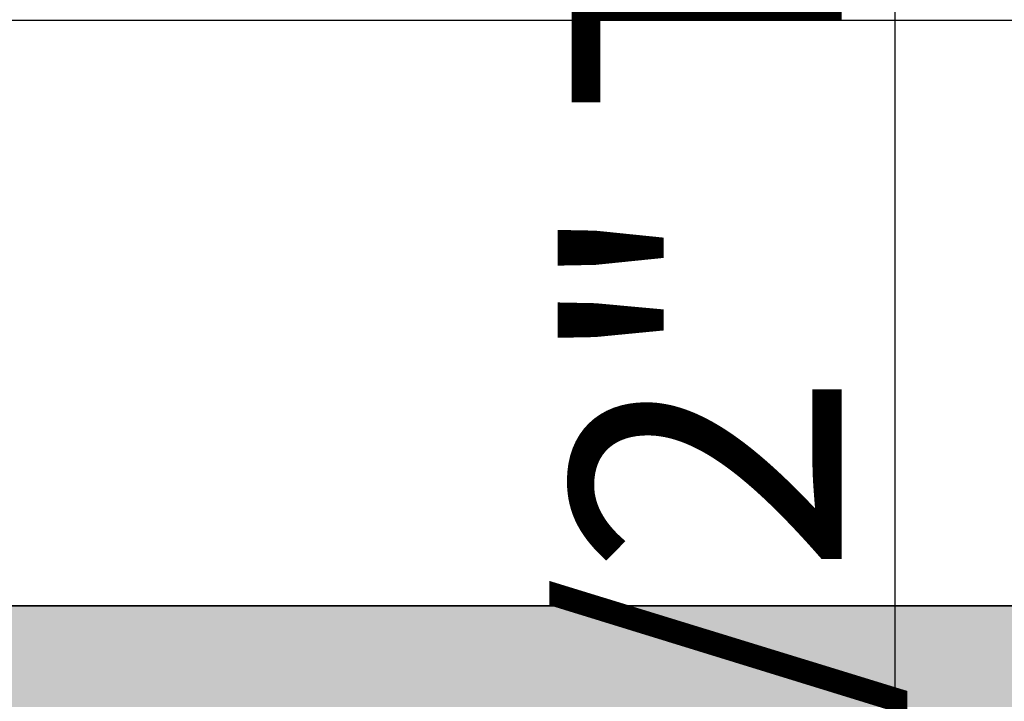
# Model space of a CAD drawing. Units: inches. Extents: x 2083 to 3317, y 1141 to 2115.
# Tile 18 of 256: x 2296 to 2340, y 1417 to 1447. Entities that reach past the tile are written whole.
import ezdxf

# ---------------------------------------------------------------- set-up
doc = ezdxf.new("R2010")
doc.units = ezdxf.units.IN
doc.layers.add('A-ANNO-DIMS', color=2, linetype='Continuous', lineweight=18)
doc.layers.add('A-WALL', color=7, linetype='Continuous', lineweight=35)
doc.layers.add('A-WALL-PATT', color=251, linetype='Continuous', lineweight=13, true_color=0x636466)
doc.styles.get("Standard").update_dxf_attribs({"font": 'arial.ttf'})
doc.dimstyles.new('ISO-25', dxfattribs={"dimtxt": 12, "dimasz": 12, "dimexe": 1.25, "dimexo": 0.625, "dimtad": 1, "dimlunit": 3, "dimtxsty": 'Standard', "dimcen": 2.5, "dimadec": 0, "dimazin": 0, "dimtfac": 1, "dimtmove": 0, "dimatfit": 3, "dimfxl": 1, "dimarcsym": 0})

# ---------------------------------------------------------------- blocks, each defined once
blk = doc.blocks.new('*D22')
at = {"layer": 'A-ANNO-DIMS', "color": 0, "lineweight": -2, "transparency": 16777216}
for p, q in [((2235.96, 1362.739), (2235.96, 1376.309)), ((2322.26, 1362.739), (2322.26, 1376.309)), ((2235.96, 1375.059), (2083.007, 1375.059)), ((2310.26, 1375.059), (2247.96, 1375.059))]:
    blk.add_line(p, q, dxfattribs=at)
at = {"layer": 'A-ANNO-DIMS', "color": 0, "transparency": 16777216}
for points in [[(2247.96, 1377.059), (2247.96, 1373.059), (2235.96, 1375.059)], [(2310.26, 1377.059), (2310.26, 1373.059), (2322.26, 1375.059)]]:
    blk.add_solid(points, dxfattribs=at)
at = {"layer": 'Defpoints', "color": 0, "transparency": 16777216}
for p in [(2235.96, 1375.059), (2235.96, 1362.114), (2322.26, 1362.114)]:
    blk.add_point(p, dxfattribs=at)
at = {"layer": 'A-ANNO-DIMS', "color": 0, "transparency": 16777216, "insert": (2153.483, 1381.889), "char_height": 12, "attachment_point": 5}
blk.add_mtext('BED 7\'-2 1/2" TYP.', dxfattribs=at)
blk = doc.blocks.new('*D23')
at = {"layer": 'A-ANNO-DIMS', "color": 0, "lineweight": -2, "transparency": 16777216}
for p, q in [((2335.205, 1362.114), (2335.205, 1476.472)), ((2322.885, 1362.114), (2336.455, 1362.114)), ((2335.205, 1306.473), (2335.205, 1350.114)), ((2322.885, 1294.473), (2336.455, 1294.473))]:
    blk.add_line(p, q, dxfattribs=at)
at = {"layer": 'A-ANNO-DIMS', "color": 0, "transparency": 16777216}
for points in [[(2333.205, 1350.114), (2337.205, 1350.114), (2335.205, 1362.114)], [(2333.205, 1306.473), (2337.205, 1306.473), (2335.205, 1294.473)]]:
    blk.add_solid(points, dxfattribs=at)
at = {"layer": 'Defpoints', "color": 0, "transparency": 16777216}
for p in [(2322.26, 1362.114), (2335.205, 1362.114), (2322.26, 1294.473)]:
    blk.add_point(p, dxfattribs=at)
at = {"layer": 'A-ANNO-DIMS', "color": 0, "transparency": 16777216, "insert": (2328.376, 1425.293), "char_height": 12, "attachment_point": 5, "rotation": 90}
blk.add_mtext('5\'-7 1/2" TYP.', dxfattribs=at)
blk = doc.blocks.new('*D30')
at = {"layer": 'A-ANNO-DIMS', "color": 0, "lineweight": -2, "transparency": 16777216}
for p, q in [((2240.018, 1445.274), (2240.018, 1448.046)), ((2254.329, 1445.274), (2254.329, 1448.046)), ((2228.018, 1446.796), (2216.018, 1446.796)), ((2240.018, 1446.796), (2254.329, 1446.796)), ((2266.329, 1446.796), (2413.765, 1446.796))]:
    blk.add_line(p, q, dxfattribs=at)
at = {"layer": 'A-ANNO-DIMS', "color": 0, "transparency": 16777216}
for points in [[(2228.018, 1448.796), (2228.018, 1444.796), (2240.018, 1446.796)], [(2266.329, 1448.796), (2266.329, 1444.796), (2254.329, 1446.796)]]:
    blk.add_solid(points, dxfattribs=at)
at = {"layer": 'Defpoints', "color": 0, "transparency": 16777216}
for p in [(2254.329, 1446.796), (2240.018, 1444.649), (2254.329, 1444.649)]:
    blk.add_point(p, dxfattribs=at)
at = {"layer": 'A-ANNO-DIMS', "color": 0, "transparency": 16777216, "insert": (2346.047, 1453.625), "char_height": 12, "attachment_point": 5}
blk.add_mtext('WC 1\'-2 1/2" TYP.', dxfattribs=at)

msp = doc.modelspace()

# ---------------------------------------------------------------- hatches: boundary and pattern name
at = {"layer": 'A-WALL-PATT'}
h = msp.add_hatch(color=256, dxfattribs=at)
h.dxf.hatch_style = 1
h.paths.add_polyline_path([(3126.96, 2020.761), (2748.96, 2020.761), (2604.96, 2020.761), (2226.96, 2020.761), (2226.96, 1702.761), (2466.96, 1702.761), (2466.96, 1582.761), (2418.96, 1582.761), (2418.96, 1477.761), (2226.96, 1477.761), (2226.96, 1263.261), (2544.96, 1263.261), (2544.96, 1411.761), (2604.96, 1411.761), (2685.96, 1411.761), (2685.96, 1420.761), (2604.96, 1420.761), (2604.96, 1573.761), (2604.96, 1702.761), (2604.96, 2011.761), (2748.96, 2011.761), (2748.96, 1702.761), (2862.96, 1702.761), (2862.96, 1621.761), (2871.96, 1621.761), (2871.96, 1702.761), (2883.96, 1702.761), (2883.96, 1706.939, -0.026459), (2883.96, 1711.761), (2757.96, 1711.761), (2757.96, 1807.761), (2787.96, 1807.761), (2787.96, 1812.261), (2757.96, 1812.261), (2757.96, 2011.761), (2877.96, 2011.761), (2877.96, 1812.261), (2847.96, 1812.261), (2847.96, 1807.761), (2889.836, 1807.761), (2889.836, 1812.261), (2882.46, 1812.261), (2882.46, 2011.761), (3117.96, 2011.761), (3117.96, 1812.261), (2937.836, 1812.261), (2937.836, 1807.761), (2995.71, 1807.761), (2995.71, 1796.118), (3000.21, 1796.118), (3000.21, 1807.761), (3117.96, 1807.761), (3117.96, 1711.761), (3000.21, 1711.761), (3000.21, 1760.118), (2998.573, 1760.118, -0.020711), (2995.71, 1760.118), (2995.71, 1711.761), (2931.96, 1711.761), (2931.96, 1702.761), (3126.96, 1702.761)])
h.paths.add_polyline_path([(2471.46, 2011.761), (2471.46, 1810.011), (2462.717, 1810.011), (2462.717, 1805.511), (2505.96, 1805.511), (2505.96, 1810.011), (2475.96, 1810.011), (2475.96, 2011.761), (2595.96, 2011.761), (2595.96, 1810.011), (2565.96, 1810.011), (2565.96, 1805.511), (2595.96, 1805.511), (2595.96, 1711.761), (2235.96, 1711.761), (2235.96, 1805.511), (2353.71, 1805.511), (2353.71, 1796.054), (2358.21, 1796.054), (2358.21, 1805.511), (2414.717, 1805.511), (2414.717, 1810.011), (2235.96, 1810.011), (2235.96, 2011.761)], flags=16)
h.paths.add_polyline_path([(2270.205, 1994.61), (2270.205, 1970.61), (2246.205, 1970.61), (2246.205, 1994.61)], flags=0)
edge = h.paths.add_edge_path(flags=0)
edge.add_ellipse((2332.027, 1899.798), major_axis=(-3.043, 3.043), ratio=0.168252, start_angle=-161.3322, end_angle=-156.3071, ccw=False)
edge.add_ellipse((2333.082, 1898.744), major_axis=(-1.055, 1.055), ratio=0.453532, start_angle=-123.371, end_angle=-94.1591)
edge = h.paths.add_edge_path(flags=0)
edge.add_ellipse((2332.027, 1968.876), major_axis=(3.043, 3.043), ratio=0.168252, start_angle=18.6678, end_angle=23.6929)
edge.add_spline(control_points=[(2332.926, 1970.691), (2332.227, 1970.336), (2330.894, 1969.659), (2328.413, 1970.932), (2327.204, 1967.749), (2324.71, 1969.956), (2322.533, 1967.012), (2320.013, 1971.296), (2317.68, 1968.158), (2316.041, 1967.102), (2315.427, 1966.81)], knot_values=[0, 0, 0, 0, 2.267059, 4.324559, 6.685584, 8.878641, 11.121502, 14.300359, 17.755284, 19.732645, 19.732645, 19.732645, 19.732645], degree=3, periodic=0)
edge.add_ellipse((2332.027, 1968.876), major_axis=(3.043, 3.043), ratio=0.168252, start_angle=18.6678, end_angle=23.6929, ccw=False)
edge.add_ellipse((2333.082, 1969.931), major_axis=(1.055, 1.055), ratio=0.453532, start_angle=56.629, end_angle=85.8409, ccw=False)
edge = h.paths.add_edge_path(flags=0)
edge.add_spline(control_points=[(2296.428, 1967.988), (2293.628, 1965.336), (2287.704, 1959.727), (2299.744, 1949.996), (2294.533, 1935.669), (2290.573, 1920.604), (2293.394, 1909.974), (2296.185, 1904.967)], knot_values=[0.099185, 0.099185, 0.099185, 0.099185, 0.345301, 0.619822, 0.982653, 1.386093, 1.810555, 1.810555, 1.810555, 1.810555], degree=3, periodic=0)
edge.add_spline(control_points=[(2296.185, 1904.967), (2297.384, 1902.619), (2298.001, 1901.949), (2298.553, 1901.468)], knot_values=[0.006246, 0.006246, 0.006246, 0.006246, 0.055476, 0.055476, 0.055476, 0.055476], degree=3, periodic=0)
edge.add_spline(control_points=[(2298.553, 1901.468), (2297.259, 1900.923), (2295.225, 1900.232), (2293.06, 1900.614), (2292.101, 1900.788), (2292.09, 1900.791)], knot_values=[0.312835, 0.312835, 0.312835, 0.312835, 0.40178, 0.474987, 0.475903, 0.475903, 0.475903, 0.475903], degree=3, periodic=0)
edge.add_arc((2292.794, 1904.664), 3.937, 215.4209, 259.6982, ccw=False)
edge.add_spline(control_points=[(2289.585, 1902.382), (2289.477, 1902.535), (2289.368, 1902.688), (2289.261, 1902.841)], knot_values=[0.102872, 0.102872, 0.102872, 0.102872, 0.116896, 0.116896, 0.116896, 0.116896], degree=3, periodic=0)
edge.add_spline(control_points=[(2289.261, 1902.841), (2288.687, 1902.55), (2287.64, 1902.02), (2285.881, 1901.874), (2283.853, 1901.504), (2281.72, 1899.711), (2278.467, 1899.493), (2276.157, 1901.883), (2272.259, 1899.804), (2267.778, 1901.843), (2262.244, 1900.184), (2257.415, 1901.782), (2254.318, 1900.726), (2253.178, 1900.337)], knot_values=[0, 0, 0, 0, 1.907977, 3.477176, 5.261074, 7.972851, 11.680248, 13.717921, 16.939592, 22.789562, 27.502503, 33.595215, 37.145618, 37.145618, 37.145618, 37.145618], degree=3, periodic=0)
edge.add_line((2253.178, 1900.337), (2250.244, 1902.841))
edge.add_line((2250.244, 1902.841), (2250.244, 1965.833))
edge.add_line((2250.244, 1965.833), (2253.178, 1968.337))
edge.add_spline(control_points=[(2253.178, 1968.337), (2254.318, 1967.948), (2257.415, 1966.892), (2262.244, 1968.49), (2267.778, 1966.831), (2271.527, 1968.537), (2273.876, 1967.828), (2274.207, 1967.728)], knot_values=[0, 0, 0, 0, 0.09018, 0.244935, 0.364644, 0.513233, 0.537855, 0.537855, 0.537855, 0.537855], degree=3, periodic=0)
edge.add_arc((2274.353, 1963.793), 3.937, 72.0511, 92.1279, ccw=False)
edge.add_arc((2281.297, 1985.23), 18.596, 252.0511, 288.5657)
edge.add_arc((2292.317, 1956.029), 12.646, 71.0268, 113.7782, ccw=False)
edge = h.paths.add_edge_path(flags=0)
edge.add_spline(control_points=[(2274.899, 1951.856), (2275.066, 1951.617), (2275.233, 1951.377), (2275.398, 1951.136)], knot_values=[1.409916, 1.409916, 1.409916, 1.409916, 1.43159, 1.43159, 1.43159, 1.43159], degree=3, periodic=0)
edge.add_spline(control_points=[(2275.398, 1951.136), (2275.792, 1950.562), (2276.179, 1949.984), (2276.546, 1949.397)], knot_values=[1.358238, 1.358238, 1.358238, 1.358238, 1.409916, 1.409916, 1.409916, 1.409916], degree=3, periodic=0)
edge.add_line((2276.546, 1949.397), (2277.437, 1947.862))
edge.add_spline(control_points=[(2277.437, 1947.862), (2276.304, 1945.673), (2274.64, 1942.427), (2274.632, 1938.094), (2272.799, 1930.852), (2274.356, 1943.897), (2275.948, 1947.923), (2276.546, 1949.397)], knot_values=[0.005632, 0.005632, 0.005632, 0.005632, 0.186014, 0.266002, 0.357087, 0.59639, 0.739732, 0.739732, 0.739732, 0.739732], degree=3, periodic=0)
edge.add_spline(control_points=[(2276.546, 1949.397), (2276.179, 1949.984), (2275.792, 1950.562), (2275.398, 1951.136)], knot_values=[1.358238, 1.358238, 1.358238, 1.358238, 1.409916, 1.409916, 1.409916, 1.409916], degree=3, periodic=0)
edge.add_spline(control_points=[(2275.398, 1951.136), (2274.943, 1950.08), (2274.208, 1948.025), (2273.935, 1944.851), (2272.469, 1937.627), (2273.466, 1945.696), (2274.701, 1951.059), (2274.899, 1951.856)], knot_values=[0.104364, 0.104364, 0.104364, 0.104364, 0.189636, 0.269624, 0.36071, 0.600013, 0.644622, 0.644622, 0.644622, 0.644622], degree=3, periodic=0)
h.paths.add_polyline_path([(2269.168, 1963.128, -0.357527), (2268.171, 1960.976, -0.092561), (2268.171, 1939.436, -0.357527), (2269.168, 1937.285, -0.357527), (2267.016, 1938.282, -0.164785), (2254.686, 1938.282, -0.357527), (2252.534, 1937.285, -0.357527), (2253.531, 1939.436, -0.092561), (2253.531, 1960.976, -0.357527), (2252.534, 1963.128, -0.357527), (2254.686, 1962.131, -0.164785), (2267.016, 1962.131, -0.357527)], flags=0)
h.paths.add_polyline_path([(2248.874, 1967.802), (2248.874, 1957.028), (2249.458, 1957.028), (2249.458, 1911.647), (2248.874, 1911.647), (2248.874, 1900.873), (2246.512, 1900.873, 0.197327), (2244.15, 1902.457), (2244.15, 1966.218, 0.197327), (2246.512, 1967.802)], flags=0)
h.paths.add_polyline_path([(2269.168, 1931.389, -0.357527), (2268.171, 1929.238, -0.092561), (2268.171, 1907.698, -0.357527), (2269.168, 1905.547, -0.357527), (2267.016, 1906.544, -0.164785), (2254.686, 1906.544, -0.357527), (2252.534, 1905.547, -0.357527), (2253.531, 1907.698, -0.092561), (2253.531, 1929.238, -0.357527), (2252.534, 1931.389, -0.357527), (2254.686, 1930.392, -0.164785), (2267.016, 1930.392, -0.357527)], flags=0)
edge = h.paths.add_edge_path(flags=0)
edge.add_spline(control_points=[(2276.197, 1906.724), (2276.168, 1909.029), (2276.114, 1913.372), (2270.598, 1924.925), (2273.905, 1919.013), (2275.922, 1916.262), (2275.475, 1912.402), (2277.258, 1910.381), (2276.696, 1908.225), (2276.646, 1906.813), (2276.618, 1906.008)], knot_values=[0, 0, 0, 0, 8.61026, 16.221274, 18.843057, 23.804898, 27.440828, 29.356102, 31.203478, 33.650687, 33.650687, 33.650687, 33.650687], degree=3, periodic=0)
edge.add_spline(control_points=[(2276.618, 1906.008), (2276.623, 1905.624), (2276.498, 1904.629), (2275.442, 1903.855), (2274.937, 1903.08), (2274.859, 1902.841)], knot_values=[0.156488, 0.156488, 0.156488, 0.156488, 0.184398, 0.231376, 0.250598, 0.250598, 0.250598, 0.250598], degree=3, periodic=0)
edge.add_line((2274.859, 1902.841), (2276.506, 1902.841))
edge.add_spline(control_points=[(2276.506, 1902.841), (2276.788, 1903.085), (2277.665, 1904.125), (2278.25, 1904.341), (2277.654, 1908.527), (2278.156, 1906.228), (2278.1, 1905.286), (2278.847, 1904.069), (2277.857, 1903.415), (2277.874, 1902.991), (2277.904, 1902.841)], knot_values=[0.059574, 0.059574, 0.059574, 0.059574, 0.080753, 0.103741, 0.16972, 0.176036, 0.207137, 0.240474, 0.262341, 0.27366, 0.27366, 0.27366, 0.27366], degree=3, periodic=0)
edge.add_line((2277.904, 1902.841), (2280.03, 1902.841))
edge.add_spline(control_points=[(2280.03, 1902.841), (2279.888, 1903.088), (2279.499, 1903.982), (2280.152, 1905.939), (2278.104, 1909.658), (2279.762, 1907.185), (2280.328, 1904.875), (2280.485, 1903.49), (2281.463, 1903.249), (2281.758, 1902.936), (2281.834, 1902.841)], knot_values=[0.013856, 0.013856, 0.013856, 0.013856, 0.034874, 0.088867, 0.107879, 0.126738, 0.158714, 0.193757, 0.217487, 0.226722, 0.226722, 0.226722, 0.226722], degree=3, periodic=0)
edge.add_spline(control_points=[(2281.834, 1902.841), (2281.788, 1902.827), (2281.647, 1902.783), (2281.396, 1902.859), (2281.088, 1902.985), (2280.721, 1903.061), (2280.333, 1903.026), (2280.125, 1902.899), (2280.03, 1902.841)], knot_values=[0, 0, 0, 0, 0.14413, 0.435517, 0.749276, 1.153046, 1.548371, 1.878348, 1.878348, 1.878348, 1.878348], degree=3, periodic=0)
edge.add_line((2280.03, 1902.841), (2277.904, 1902.841))
edge.add_spline(control_points=[(2277.904, 1902.841), (2277.893, 1902.796), (2277.865, 1902.68), (2277.607, 1902.687), (2277.274, 1902.801), (2276.838, 1902.62), (2276.584, 1902.789), (2276.506, 1902.841)], knot_values=[0, 0, 0, 0, 0.127189, 0.326199, 0.628009, 1.24357, 1.515331, 1.515331, 1.515331, 1.515331], degree=3, periodic=0)
edge.add_line((2276.506, 1902.841), (2274.859, 1902.841))
edge.add_spline(control_points=[(2274.859, 1902.841), (2274.814, 1902.899), (2274.725, 1903.013), (2274.493, 1903.119), (2274.244, 1902.961), (2273.937, 1903.185), (2273.614, 1902.983), (2273.408, 1902.883), (2273.322, 1902.841)], knot_values=[0, 0, 0, 0, 0.21843, 0.436957, 0.687977, 0.990379, 1.398396, 1.69185, 1.69185, 1.69185, 1.69185], degree=3, periodic=0)
edge.add_spline(control_points=[(2273.322, 1902.841), (2273.617, 1903.446), (2274.274, 1904.538), (2276.027, 1904.574), (2276.207, 1906.584), (2276.197, 1906.724)], knot_values=[0.012227, 0.012227, 0.012227, 0.012227, 0.059472, 0.106218, 0.134458, 0.134458, 0.134458, 0.134458], degree=3, periodic=0)
h.paths.add_polyline_path([(2270.776, 1897.79), (2270.776, 1873.79), (2246.776, 1873.79), (2246.776, 1897.79)], flags=0)
h.paths.add_polyline_path([(2353.71, 1760.005), (2353.71, 1760.054), (2358.21, 1760.054, -0.033729)], flags=0)
h.paths.add_polyline_path([(2321.819, 1737.529), (2341.995, 1737.529, -0.414214), (2343.203, 1736.321), (2343.203, 1721.021, -0.414214), (2341.995, 1719.813), (2321.819, 1719.813, -0.414214), (2320.611, 1721.021), (2320.611, 1736.321, -0.414214)], flags=0)
h.paths.add_polyline_path([(2324.235, 1736.321), (2339.579, 1736.321, -0.414214), (2341.995, 1733.905), (2341.995, 1725.45, -0.414214), (2339.579, 1723.034), (2333.681, 1723.034), (2333.845, 1722.045, -0.870646), (2335.425, 1721.826, -0.767327), (2333.923, 1721.423), (2331.291, 1721.423, -0.767327), (2329.788, 1721.826, -0.870646), (2331.368, 1722.045), (2331.533, 1723.034), (2324.235, 1723.034, -0.414214), (2321.819, 1725.45), (2321.819, 1733.905, -0.414214)], flags=0)
h.paths.add_polyline_path([(2570.484, 1928.615), (2589.684, 1928.615), (2590.169, 1928.615), (2590.169, 1904.993), (2570.484, 1904.993)], flags=0)
h.paths.add_polyline_path([(2574.447, 1927.264, -1), (2572.829, 1927.264, -1)], flags=0)
h.paths.add_polyline_path([(2573.09, 1926.941), (2573.925, 1927.776), (2574.148, 1927.553), (2573.313, 1926.718)], flags=0)
h.paths.add_polyline_path([(2578.779, 1919.73, -1), (2571.592, 1919.73, -1)], flags=0)
h.paths.add_polyline_path([(2578.385, 1919.73, -1), (2571.985, 1919.73, -1)], flags=0)
h.paths.add_polyline_path([(2331.596, 1729.476, -1), (2333.618, 1729.476, -1)], flags=0)
h.paths.add_polyline_path([(2578.034, 1927.264, -1), (2576.416, 1927.264, -1)], flags=0)
h.paths.add_polyline_path([(2576.689, 1927.531), (2576.912, 1927.754), (2577.747, 1926.919), (2577.524, 1926.696)], flags=0)
h.paths.add_polyline_path([(2578.139, 1909.86, -1), (2572.232, 1909.86, -1)], flags=0)
h.paths.add_polyline_path([(2577.745, 1909.86, -1), (2572.625, 1909.86, -1)], flags=0)
h.paths.add_polyline_path([(2583.798, 1927.264, -1), (2582.179, 1927.264, -1)], flags=0)
h.paths.add_polyline_path([(2582.719, 1927.754), (2583.554, 1926.919), (2583.331, 1926.696), (2582.496, 1927.531)], flags=0)
h.paths.add_polyline_path([(2582.496, 1927.531), (2582.719, 1927.754), (2583.554, 1926.919), (2583.331, 1926.696)], flags=0)
h.paths.add_polyline_path([(2587.739, 1920.53, -1), (2581.832, 1920.53, -1)], flags=0)
h.paths.add_polyline_path([(2587.345, 1920.53, -1), (2582.225, 1920.53, -1)], flags=0)
h.paths.add_polyline_path([(2587.385, 1927.264, -1), (2585.766, 1927.264, -1)], flags=0)
h.paths.add_polyline_path([(2586.082, 1926.98), (2586.917, 1927.815), (2587.14, 1927.593), (2586.305, 1926.758)], flags=0)
h.paths.add_polyline_path([(2588.379, 1910.66, -1), (2581.192, 1910.66, -1)], flags=0)
h.paths.add_polyline_path([(2587.985, 1910.66, -1), (2581.585, 1910.66, -1)], flags=0)
h.paths.add_polyline_path([(2417.168, 1729.478), (2437.344, 1729.478, -0.414214), (2438.552, 1728.27), (2438.552, 1712.969, -0.414214), (2437.344, 1711.761), (2417.168, 1711.761, -0.414214), (2415.96, 1712.969), (2415.96, 1728.27, -0.414214)], flags=0)
h.paths.add_polyline_path([(2419.584, 1728.27), (2434.928, 1728.27, -0.414214), (2437.344, 1725.854), (2437.344, 1717.398, -0.414214), (2434.928, 1714.983), (2429.029, 1714.983), (2429.194, 1713.994, -0.870646), (2430.774, 1713.775, -0.767327), (2429.271, 1713.372), (2426.64, 1713.372, -0.767327), (2425.137, 1713.775, -0.870646), (2426.717, 1713.994), (2426.882, 1714.983), (2419.584, 1714.983, -0.414214), (2417.168, 1717.398), (2417.168, 1725.854, -0.414214)], flags=0)
h.paths.add_polyline_path([(2419.584, 1728.27), (2434.928, 1728.27, -0.414214), (2437.344, 1725.854), (2437.344, 1717.398, -0.414214), (2434.928, 1714.983), (2429.029, 1714.983), (2428.358, 1719.009), (2427.553, 1719.009), (2426.882, 1714.983), (2419.584, 1714.983, -0.414214), (2417.168, 1717.398), (2417.168, 1725.854, -0.414214)], flags=0)
h.paths.add_polyline_path([(2426.944, 1721.425, -1), (2428.967, 1721.425, -1)], flags=0)
h.paths.add_polyline_path([(2475.96, 1702.761), (2595.96, 1702.761), (2595.96, 1582.761), (2475.96, 1582.761)], flags=16)
h.paths.add_polyline_path([(2427.96, 1573.761), (2595.96, 1573.761), (2595.96, 1468.761), (2595.96, 1420.761), (2384.46, 1420.761), (2384.46, 1468.761), (2427.96, 1468.761)], flags=16)
h.paths.add_polyline_path([(2379.96, 1468.761), (2379.96, 1420.761), (2235.96, 1420.761), (2235.96, 1468.761)], flags=16)
h.paths.add_polyline_path([(2317.816, 1466.696), (2337.992, 1466.696, -0.414214), (2339.2, 1465.488), (2339.2, 1450.187, -0.414214), (2337.992, 1448.979), (2317.816, 1448.979, -0.414214), (2316.608, 1450.187), (2316.608, 1465.488, -0.414214)], flags=0)
h.paths.add_polyline_path([(2320.232, 1465.488), (2335.576, 1465.488, -0.414214), (2337.992, 1463.072), (2337.992, 1454.616, -0.414214), (2335.576, 1452.2), (2329.677, 1452.2), (2329.842, 1451.212, -0.870646), (2331.422, 1450.992, -0.767327), (2329.92, 1450.59), (2327.288, 1450.59, -0.767327), (2325.785, 1450.992, -0.870646), (2327.365, 1451.212), (2327.53, 1452.2), (2320.232, 1452.2, -0.414214), (2317.816, 1454.616), (2317.816, 1463.072, -0.414214)], flags=0)
h.paths.add_polyline_path([(2320.232, 1465.488), (2335.576, 1465.488, -0.414214), (2337.992, 1463.072), (2337.992, 1454.616, -0.414214), (2335.576, 1452.2), (2329.677, 1452.2), (2329.006, 1456.227), (2328.201, 1456.227), (2327.53, 1452.2), (2320.232, 1452.2, -0.414214), (2317.816, 1454.616), (2317.816, 1463.072, -0.414214)], flags=0)
h.paths.add_polyline_path([(2327.593, 1458.643, -1), (2329.615, 1458.643, -1)], flags=0)
h.paths.add_polyline_path([(2244.412, 1433.34), (2241.921, 1433.34, -0.414214), (2240.018, 1435.244), (2240.018, 1440.953, -0.414211), (2241.921, 1442.856), (2244.412, 1442.856, -1.976472)], flags=0)
h.paths.add_polyline_path([(2245.357, 1434.398, -0.414214), (2245.357, 1441.799, -2.144098)], flags=0)
h.paths.add_polyline_path([(2535.96, 1416.261), (2535.96, 1272.261), (2235.96, 1272.261), (2235.96, 1416.261)], flags=16)
h.paths.add_polyline_path([(2260.12, 1384.293), (2260.12, 1362.039), (2237.865, 1362.039), (2237.865, 1384.293)], flags=0)
edge = h.paths.add_edge_path(flags=0)
edge.add_line((2318.252, 1362.093), (2318.146, 1362.001))
edge.add_ellipse((2317.445, 1360.431), major_axis=(2.822, 2.822), ratio=0.168252, start_angle=18.6678, end_angle=20.9481, ccw=False)
edge.add_ellipse((2318.423, 1361.409), major_axis=(0.978, 0.978), ratio=0.453532, start_angle=56.629, end_angle=70.2262, ccw=False)
edge = h.paths.add_edge_path(flags=0)
edge.add_line((2319.107, 1295.571), (2319.015, 1295.677))
edge.add_ellipse((2317.445, 1296.378), major_axis=(-2.822, 2.822), ratio=0.168252, start_angle=-161.3322, end_angle=-159.0519, ccw=False)
edge.add_ellipse((2318.423, 1295.4), major_axis=(-0.978, 0.978), ratio=0.453532, start_angle=-123.371, end_angle=-109.7738)
edge = h.paths.add_edge_path(flags=0)
edge.add_spline(control_points=[(2284.21, 1301.17), (2284.581, 1300.445), (2284.891, 1299.892), (2285.16, 1299.461)], knot_values=[0.039066, 0.039066, 0.039066, 0.039066, 0.055476, 0.055476, 0.055476, 0.055476], degree=3, periodic=0)
edge.add_line((2285.16, 1299.461), (2284.21, 1301.17))
edge = h.paths.add_edge_path(flags=0)
edge.add_line((2280.412, 1297.298), (2283.37, 1297.036))
edge.add_line((2283.37, 1297.036), (2286.406, 1297.926))
edge.add_spline(control_points=[(2286.406, 1297.926), (2285.305, 1297.463), (2284.345, 1297.129), (2283.37, 1297.036)], knot_values=[0.394369, 0.394369, 0.394369, 0.394369, 0.475903, 0.475903, 0.475903, 0.475903], degree=3, periodic=0)
edge.add_spline(control_points=[(2283.37, 1297.036), (2283.281, 1297.028), (2282.316, 1296.957), (2281.313, 1297.134), (2280.423, 1297.296), (2280.412, 1297.298)], knot_values=[0.312835, 0.312835, 0.312835, 0.312835, 0.320246, 0.393453, 0.394369, 0.394369, 0.394369, 0.394369], degree=3, periodic=0)
edge = h.paths.add_edge_path(flags=0)
edge.add_line((2284.436, 1359.607), (2280.446, 1355.328))
edge.add_line((2280.446, 1355.328), (2279.58, 1351.018))
edge.add_line((2279.58, 1351.018), (2282.413, 1346.58))
edge.add_spline(control_points=[(2282.413, 1346.58), (2283.153, 1345.589), (2284.253, 1344.029), (2284.801, 1342.387), (2284.935, 1341.806)], knot_values=[1.240098, 1.240098, 1.240098, 1.240098, 1.332892, 1.382712, 1.382712, 1.382712, 1.382712], degree=3, periodic=0)
edge.add_spline(control_points=[(2284.935, 1341.806), (2285.319, 1340.141), (2285.233, 1338.409), (2284.91, 1336.654)], knot_values=[1.097484, 1.097484, 1.097484, 1.097484, 1.240098, 1.240098, 1.240098, 1.240098], degree=3, periodic=0)
edge.add_spline(control_points=[(2284.91, 1336.654), (2284.587, 1334.899), (2284.027, 1333.12), (2283.463, 1331.361)], knot_values=[0.95487, 0.95487, 0.95487, 0.95487, 1.097484, 1.097484, 1.097484, 1.097484], degree=3, periodic=0)
edge.add_line((2283.463, 1331.361), (2281.89, 1326.153))
edge.add_line((2281.89, 1326.153), (2280.756, 1321.056))
edge.add_line((2280.756, 1321.056), (2280.299, 1316.002))
edge.add_line((2280.299, 1316.002), (2280.716, 1310.95))
edge.add_line((2280.716, 1310.95), (2282.028, 1305.972))
edge.add_line((2282.028, 1305.972), (2284.21, 1301.17))
edge.add_spline(control_points=[(2284.21, 1301.17), (2283.341, 1302.73), (2282.612, 1304.336), (2282.028, 1305.972)], knot_values=[0.099185, 0.099185, 0.099185, 0.099185, 0.241799, 0.241799, 0.241799, 0.241799], degree=3, periodic=0)
edge.add_spline(control_points=[(2282.028, 1305.972), (2281.444, 1307.608), (2281.005, 1309.273), (2280.716, 1310.95)], knot_values=[0.241799, 0.241799, 0.241799, 0.241799, 0.384413, 0.384413, 0.384413, 0.384413], degree=3, periodic=0)
edge.add_spline(control_points=[(2280.716, 1310.95), (2280.433, 1312.588), (2280.289, 1314.277), (2280.299, 1315.962), (2280.299, 1316.002)], knot_values=[0.384413, 0.384413, 0.384413, 0.384413, 0.523647, 0.527028, 0.527028, 0.527028, 0.527028], degree=3, periodic=0)
edge.add_spline(control_points=[(2280.299, 1316.002), (2280.312, 1317.687), (2280.478, 1319.368), (2280.756, 1321.056)], knot_values=[0.527028, 0.527028, 0.527028, 0.527028, 0.669642, 0.669642, 0.669642, 0.669642], degree=3, periodic=0)
edge.add_spline(control_points=[(2280.756, 1321.056), (2281.035, 1322.744), (2281.426, 1324.44), (2281.89, 1326.153)], knot_values=[0.669642, 0.669642, 0.669642, 0.669642, 0.812256, 0.812256, 0.812256, 0.812256], degree=3, periodic=0)
edge.add_spline(control_points=[(2281.89, 1326.153), (2282.264, 1327.533), (2282.788, 1329.262), (2283.353, 1331.018), (2283.463, 1331.361)], knot_values=[0.812256, 0.812256, 0.812256, 0.812256, 0.927087, 0.95487, 0.95487, 0.95487, 0.95487], degree=3, periodic=0)
edge.add_line((2283.463, 1331.361), (2284.91, 1336.654))
edge.add_line((2284.91, 1336.654), (2284.935, 1341.806))
edge.add_line((2284.935, 1341.806), (2282.413, 1346.58))
edge.add_spline(control_points=[(2282.413, 1346.58), (2281.275, 1348.104), (2280.078, 1349.57), (2279.58, 1351.018)], knot_values=[1.382712, 1.382712, 1.382712, 1.382712, 1.525326, 1.525326, 1.525326, 1.525326], degree=3, periodic=0)
edge.add_spline(control_points=[(2279.58, 1351.018), (2279.443, 1351.415), (2279.136, 1352.857), (2279.735, 1354.29), (2280.446, 1355.328)], knot_values=[1.525326, 1.525326, 1.525326, 1.525326, 1.564439, 1.667941, 1.667941, 1.667941, 1.667941], degree=3, periodic=0)
edge.add_spline(control_points=[(2280.446, 1355.328), (2281.426, 1356.758), (2282.931, 1358.183), (2284.436, 1359.607)], knot_values=[1.667941, 1.667941, 1.667941, 1.667941, 1.810555, 1.810555, 1.810555, 1.810555], degree=3, periodic=0)
edge.add_arc((2280.623, 1348.518), 11.726, 71.0268, 113.7782)
edge.add_arc((2270.405, 1375.595), 17.244, 252.0511, 288.5657, ccw=False)
edge.add_arc((2263.966, 1355.718), 3.651, 72.0511, 92.1279)
edge.add_arc((2263.966, 1355.718), 3.651, 92.1279, 177.9851)
edge.add_spline(control_points=[(2260.318, 1355.846), (2260.26, 1354.221), (2260.551, 1350.187), (2262.999, 1346.766), (2264.473, 1344.649)], knot_values=[1.43159, 1.43159, 1.43159, 1.43159, 1.564144, 1.770695, 1.770695, 1.770695, 1.770695], degree=3, periodic=0)
edge.add_line((2264.473, 1344.649), (2264.936, 1343.983))
edge.add_spline(control_points=[(2263.801, 1340.248), (2263.843, 1340.514), (2264.067, 1341.756), (2264.513, 1343.002), (2264.935, 1343.981)], knot_values=[0.53657, 0.53657, 0.53657, 0.53657, 0.559349, 0.644622, 0.644622, 0.644622, 0.644622], degree=3, periodic=0)
edge.add_spline(control_points=[(2264.935, 1343.981), (2265.118, 1343.715), (2265.299, 1343.448), (2265.477, 1343.179)], knot_values=[1.384077, 1.384077, 1.384077, 1.384077, 1.409916, 1.409916, 1.409916, 1.409916], degree=3, periodic=0)
edge.add_spline(control_points=[(2265.477, 1343.179), (2265.655, 1342.911), (2265.829, 1342.641), (2265.999, 1342.369)], knot_values=[1.358238, 1.358238, 1.358238, 1.358238, 1.384077, 1.384077, 1.384077, 1.384077], degree=3, periodic=0)
edge.add_line((2265.999, 1342.369), (2266.826, 1340.946))
edge.add_spline(control_points=[(2266.826, 1340.946), (2268.894, 1337.09), (2271.398, 1325.843), (2270.516, 1310.569), (2275.919, 1301.861), (2277.79, 1299.199)], knot_values=[0.116896, 0.116896, 0.116896, 0.116896, 0.472987, 1.050969, 1.313793, 1.313793, 1.313793, 1.313793], degree=3, periodic=0)
edge.add_spline(control_points=[(2277.79, 1299.199), (2277.839, 1299.128), (2277.889, 1299.057), (2277.94, 1298.987)], knot_values=[0.109884, 0.109884, 0.109884, 0.109884, 0.116896, 0.116896, 0.116896, 0.116896], degree=3, periodic=0)
edge.add_line((2277.94, 1298.987), (2277.789, 1299.199))
edge.add_spline(control_points=[(2277.789, 1299.199), (2277.257, 1298.929), (2276.286, 1298.438), (2275.039, 1298.334), (2274.383, 1298.239), (2274.215, 1298.209)], knot_values=[33.12187, 33.12187, 33.12187, 33.12187, 35.029056, 36.598255, 37.144827, 37.144827, 37.144827, 37.144827], degree=3, periodic=0)
edge.add_line((2274.215, 1298.209), (2273.073, 1297.893))
edge.add_spline(control_points=[(2273.073, 1297.893), (2272.323, 1297.58), (2271.039, 1296.511), (2269.248, 1296.226), (2268.423, 1296.375)], knot_values=[26.532584, 26.532584, 26.532584, 26.532584, 29.198919, 31.839101, 31.839101, 31.839101, 31.839101], degree=3, periodic=0)
edge.add_line((2268.423, 1296.375), (2263.879, 1297.458))
edge.add_spline(control_points=[(2263.879, 1297.458), (2263.556, 1297.359), (2261.86, 1296.839), (2260.239, 1297.282), (2258.933, 1297.516)], knot_values=[15.919551, 15.919551, 15.919551, 15.919551, 16.939592, 21.226067, 21.226067, 21.226067, 21.226067], degree=3, periodic=0)
edge.add_line((2258.933, 1297.516), (2254.055, 1297.329))
edge.add_spline(control_points=[(2254.055, 1297.329), (2253.756, 1297.296), (2252.114, 1297.165), (2250.462, 1297.544), (2249.13, 1297.668)], knot_values=[5.306517, 5.306517, 5.306517, 5.306517, 6.276435, 10.613034, 10.613034, 10.613034, 10.613034], degree=3, periodic=0)
edge.add_line((2249.13, 1297.668), (2244.332, 1296.878))
edge.add_line((2244.332, 1296.878), (2241.611, 1299.199))
edge.add_line((2241.611, 1299.199), (2241.611, 1357.609))
edge.add_line((2241.611, 1357.609), (2244.332, 1359.931))
edge.add_line((2244.332, 1359.931), (2252.729, 1359.543))
edge.add_spline(control_points=[(2252.729, 1359.543), (2252.871, 1359.546), (2253.306, 1359.548), (2253.74, 1359.514), (2254.032, 1359.482)], knot_values=[0.233291, 0.233291, 0.233291, 0.233291, 0.244935, 0.268927, 0.268927, 0.268927, 0.268927], degree=3, periodic=0)
edge.add_line((2254.032, 1359.482), (2259.587, 1359.416))
edge.add_spline(control_points=[(2259.587, 1359.416), (2260.677, 1359.629), (2262.073, 1359.897), (2263.524, 1359.459), (2263.83, 1359.366)], knot_values=[0.422516, 0.422516, 0.422516, 0.422516, 0.513233, 0.537855, 0.537855, 0.537855, 0.537855], degree=3, periodic=0)
edge.add_arc((2263.966, 1355.718), 3.651, 72.0511, 92.1279, ccw=False)
edge.add_arc((2270.405, 1375.595), 17.244, 252.0511, 288.5657)
edge.add_arc((2280.623, 1348.518), 11.726, 71.0268, 113.7782, ccw=False)
h.paths.add_polyline_path([(2240.341, 1359.435), (2240.341, 1349.444), (2240.882, 1349.444), (2240.882, 1307.365), (2240.341, 1307.365), (2240.341, 1297.374), (2238.15, 1297.374, 0.197327), (2235.96, 1298.843), (2235.96, 1357.966, 0.197327), (2238.15, 1359.435)], flags=0)
h.paths.add_polyline_path([(2259.158, 1355.101, -0.357527), (2258.233, 1353.106, -0.092561), (2258.233, 1333.133, -0.357527), (2259.158, 1331.138, -0.357527), (2257.163, 1332.062, -0.164785), (2245.729, 1332.062, -0.357527), (2243.735, 1331.138, -0.357527), (2244.659, 1333.133, -0.092561), (2244.659, 1353.106, -0.357527), (2243.735, 1355.101, -0.357527), (2245.729, 1354.176, -0.164785), (2257.163, 1354.176, -0.357527)], flags=0)
edge = h.paths.add_edge_path(flags=0)
edge.add_line((2265.999, 1342.369), (2266.826, 1340.946))
edge.add_line((2266.826, 1340.946), (2265.308, 1337.814))
edge.add_line((2265.308, 1337.814), (2264.358, 1334.653))
edge.add_line((2264.358, 1334.653), (2264.262, 1333.8))
edge.add_spline(control_points=[(2264.262, 1333.8), (2264.208, 1333.187), (2264.162, 1332.366), (2264.007, 1331.414), (2263.969, 1331.202)], knot_values=[0.464444, 0.464444, 0.464444, 0.464444, 0.516691, 0.531608, 0.531608, 0.531608, 0.531608], degree=3, periodic=0)
edge.add_spline(control_points=[(2263.969, 1331.202), (2263.775, 1330.119), (2263.424, 1328.791), (2263.257, 1328.531), (2263.234, 1328.515)], knot_values=[0.372682, 0.372682, 0.372682, 0.372682, 0.44885, 0.464444, 0.464444, 0.464444, 0.464444], degree=3, periodic=0)
edge.add_spline(control_points=[(2263.234, 1328.515), (2263.096, 1328.42), (2263.131, 1329.301), (2263.275, 1330.616)], knot_values=[0.280919, 0.280919, 0.280919, 0.280919, 0.372682, 0.372682, 0.372682, 0.372682], degree=3, periodic=0)
edge.add_spline(control_points=[(2263.275, 1330.616), (2263.419, 1331.93), (2263.672, 1333.677), (2263.97, 1335.315)], knot_values=[0.189157, 0.189157, 0.189157, 0.189157, 0.280919, 0.280919, 0.280919, 0.280919], degree=3, periodic=0)
edge.add_spline(control_points=[(2263.97, 1335.315), (2264.1, 1336.032), (2264.419, 1337.622), (2264.755, 1338.864), (2264.947, 1339.491)], knot_values=[0.097394, 0.097394, 0.097394, 0.097394, 0.137578, 0.189157, 0.189157, 0.189157, 0.189157], degree=3, periodic=0)
edge.add_spline(control_points=[(2264.947, 1339.491), (2265.29, 1340.606), (2265.644, 1341.494), (2265.999, 1342.369)], knot_values=[0.005632, 0.005632, 0.005632, 0.005632, 0.097394, 0.097394, 0.097394, 0.097394], degree=3, periodic=0)
h.paths.add_polyline_path([(2259.158, 1325.671, -0.357527), (2258.233, 1323.676, -0.092561), (2258.233, 1303.703, -0.357527), (2259.158, 1301.708, -0.357527), (2257.163, 1302.633, -0.164785), (2245.729, 1302.633, -0.357527), (2243.735, 1301.708, -0.357527), (2244.659, 1303.703, -0.092561), (2244.659, 1323.676, -0.357527), (2243.735, 1325.671, -0.357527), (2245.729, 1324.747, -0.164785), (2257.163, 1324.747, -0.357527)], flags=0)
edge = h.paths.add_edge_path(flags=0)
edge.add_spline(control_points=[(2261.709, 1317.311), (2261.679, 1317.418), (2261.762, 1317.389), (2262.491, 1316.09), (2262.962, 1315.301)], knot_values=[14.955861, 14.955861, 14.955861, 14.955861, 16.221274, 18.694826, 18.694826, 18.694826, 18.694826], degree=3, periodic=0)
edge.add_spline(control_points=[(2262.962, 1315.301), (2262.99, 1315.254), (2263.702, 1314.067), (2264.349, 1313.127), (2264.73, 1312.164)], knot_values=[18.694826, 18.694826, 18.694826, 18.694826, 18.843057, 22.433791, 22.433791, 22.433791, 22.433791], degree=3, periodic=0)
edge.add_spline(control_points=[(2264.73, 1312.164), (2264.876, 1311.796), (2265.177, 1310.77), (2265.143, 1309.559), (2265.248, 1308.824)], knot_values=[22.433791, 22.433791, 22.433791, 22.433791, 23.804898, 26.172756, 26.172756, 26.172756, 26.172756], degree=3, periodic=0)
edge.add_line((2265.248, 1308.824), (2265.851, 1307.172))
edge.add_spline(control_points=[(2265.851, 1307.172), (2266.065, 1306.822), (2266.384, 1306.332), (2266.424, 1305.781), (2266.42, 1305.611)], knot_values=[28.062562, 28.062562, 28.062562, 28.062562, 29.356102, 29.911721, 29.911721, 29.911721, 29.911721], degree=3, periodic=0)
edge.add_spline(control_points=[(2266.42, 1305.611), (2266.416, 1305.433), (2266.394, 1305.25), (2266.365, 1305.066)], knot_values=[29.911721, 29.911721, 29.911721, 29.911721, 30.497837, 30.497837, 30.497837, 30.497837], degree=3, periodic=0)
edge.add_line((2266.365, 1305.066), (2266.066, 1302.136))
edge.add_spline(control_points=[(2266.066, 1302.136), (2266.071, 1301.78), (2265.998, 1301.2), (2265.663, 1300.759), (2265.509, 1300.586)], knot_values=[0.156488, 0.156488, 0.156488, 0.156488, 0.184398, 0.203543, 0.203543, 0.203543, 0.203543], degree=3, periodic=0)
edge.add_line((2265.509, 1300.586), (2264.435, 1299.199))
edge.add_line((2264.435, 1299.199), (2265.962, 1299.199))
edge.add_line((2265.962, 1299.199), (2267.336, 1301.175))
edge.add_line((2267.336, 1301.175), (2267.312, 1301.986))
edge.add_spline(control_points=[(2267.312, 1301.986), (2267.261, 1302.862), (2267.16, 1303.737), (2267.271, 1303.326)], knot_values=[0.126229, 0.126229, 0.126229, 0.126229, 0.166617, 0.166617, 0.166617, 0.166617], degree=3, periodic=0)
edge.add_spline(control_points=[(2267.271, 1303.326), (2267.28, 1303.294), (2267.31, 1303.175), (2267.373, 1302.884), (2267.406, 1302.683), (2267.418, 1302.601)], knot_values=[0.166617, 0.166617, 0.166617, 0.166617, 0.16972, 0.176036, 0.180765, 0.180765, 0.180765, 0.180765], degree=3, periodic=0)
edge.add_spline(control_points=[(2267.744, 1300.988), (2267.688, 1301.151), (2267.481, 1301.657), (2267.484, 1302.145), (2267.418, 1302.601)], knot_values=[0.180765, 0.180765, 0.180765, 0.180765, 0.193767, 0.220139, 0.220139, 0.220139, 0.220139], degree=3, periodic=0)
edge.add_line((2267.418, 1302.601), (2267.744, 1300.988))
edge.add_spline(control_points=[(2267.744, 1300.988), (2267.832, 1300.732), (2267.932, 1300.31), (2267.555, 1299.975), (2267.429, 1299.829)], knot_values=[0.220139, 0.220139, 0.220139, 0.220139, 0.240474, 0.25489, 0.25489, 0.25489, 0.25489], degree=3, periodic=0)
edge.add_line((2267.429, 1299.829), (2267.258, 1299.199))
edge.add_line((2267.258, 1299.199), (2269.23, 1299.199))
edge.add_spline(control_points=[(2269.23, 1299.199), (2269.099, 1299.429), (2268.843, 1300.016), (2269.012, 1300.916), (2268.947, 1301.661)], knot_values=[0.013856, 0.013856, 0.013856, 0.013856, 0.034874, 0.067073, 0.067073, 0.067073, 0.067073], degree=3, periodic=0)
edge.add_line((2268.947, 1301.661), (2268.432, 1303.603))
edge.add_spline(control_points=[(2268.432, 1303.603), (2268.176, 1304.192), (2267.596, 1305.251), (2268.041, 1304.623), (2268.251, 1304.282)], knot_values=[0.090155, 0.090155, 0.090155, 0.090155, 0.107879, 0.120289, 0.120289, 0.120289, 0.120289], degree=3, periodic=0)
edge.add_spline(control_points=[(2268.251, 1304.282), (2268.361, 1304.105), (2269.058, 1302.918), (2269.383, 1301.59), (2269.521, 1300.776), (2269.575, 1300.556)], knot_values=[0.120289, 0.120289, 0.120289, 0.120289, 0.126738, 0.158714, 0.173506, 0.173506, 0.173506, 0.173506], degree=3, periodic=0)
edge.add_line((2269.575, 1300.556), (2270.686, 1299.421))
edge.add_spline(control_points=[(2270.686, 1299.421), (2270.767, 1299.357), (2270.838, 1299.281), (2270.903, 1299.199)], knot_values=[0.21816, 0.21816, 0.21816, 0.21816, 0.226722, 0.226722, 0.226722, 0.226722], degree=3, periodic=0)
edge.add_line((2270.937, 1299.193), (2270.903, 1299.199))
edge.add_spline(control_points=[(2270.903, 1299.199), (2270.86, 1299.186), (2270.73, 1299.146), (2270.496, 1299.216), (2270.272, 1299.308), (2270.121, 1299.348), (2270.063, 1299.36)], knot_values=[0.939174, 0.939174, 0.939174, 0.939174, 1.083304, 1.374691, 1.68845, 1.878348, 1.878348, 1.878348, 1.878348], degree=3, periodic=0)
edge.add_line((2270.063, 1299.36), (2269.23, 1299.199))
edge.add_line((2269.23, 1299.199), (2267.258, 1299.199))
edge.add_spline(control_points=[(2267.258, 1299.199), (2267.248, 1299.157), (2267.223, 1299.05), (2266.984, 1299.057), (2266.809, 1299.116), (2266.677, 1299.109), (2266.637, 1299.105)], knot_values=[0.757665, 0.757665, 0.757665, 0.757665, 0.884854, 1.083864, 1.385675, 1.515331, 1.515331, 1.515331, 1.515331], degree=3, periodic=0)
edge.add_spline(control_points=[(2266.637, 1299.105), (2266.485, 1299.089), (2266.236, 1299.017), (2266.035, 1299.151), (2265.962, 1299.199)], knot_values=[0, 0, 0, 0, 0.485905, 0.757665, 0.757665, 0.757665, 0.757665], degree=3, periodic=0)
edge.add_line((2265.962, 1299.199), (2264.435, 1299.199))
edge.add_line((2264.435, 1299.199), (2263.858, 1299.367))
edge.add_spline(control_points=[(2263.858, 1299.367), (2263.819, 1299.371), (2263.78, 1299.386), (2263.74, 1299.402)], knot_values=[0.845925, 0.845925, 0.845925, 0.845925, 0.978627, 0.978627, 0.978627, 0.978627], degree=3, periodic=0)
edge.add_line((2263.722, 1299.396), (2263.01, 1299.199))
edge.add_spline(control_points=[(2263.01, 1299.199), (2263.246, 1299.683), (2263.506, 1300.128), (2263.873, 1300.408)], knot_values=[0.012227, 0.012227, 0.012227, 0.012227, 0.052971, 0.052971, 0.052971, 0.052971], degree=3, periodic=0)
edge.add_spline(control_points=[(2263.873, 1300.408), (2263.932, 1300.453), (2264.084, 1300.553), (2264.255, 1300.624), (2264.36, 1300.665)], knot_values=[0.052971, 0.052971, 0.052971, 0.052971, 0.059472, 0.069086, 0.069086, 0.069086, 0.069086], degree=3, periodic=0)
edge.add_line((2264.36, 1300.665), (2265.142, 1301.078))
edge.add_line((2265.142, 1301.078), (2265.676, 1302.8))
edge.add_line((2265.676, 1302.8), (2265.541, 1305.704))
edge.add_line((2265.541, 1305.704), (2264.803, 1309.328))
edge.add_line((2264.803, 1309.328), (2263.041, 1314.092))
edge.add_spline(control_points=[(2263.041, 1314.092), (2262.384, 1315.671), (2261.796, 1316.998), (2261.709, 1317.311)], knot_values=[11.216896, 11.216896, 11.216896, 11.216896, 14.955861, 14.955861, 14.955861, 14.955861], degree=3, periodic=0)
h.paths.add_polyline_path([(2871.96, 1416.261), (2895.91, 1416.261), (2895.91, 1420.761), (2871.96, 1420.761), (2871.96, 1501.761), (2862.96, 1501.761), (2862.96, 1420.761), (2805.96, 1420.761), (2805.96, 1411.761), (2862.96, 1411.761), (2862.96, 1263.261), (3126.96, 1263.261), (3126.96, 1411.761), (3126.96, 1486.761), (2943.96, 1486.761), (2943.96, 1477.761), (2967.86, 1477.761), (2967.86, 1420.761), (2943.91, 1420.761), (2943.91, 1416.261), (3117.96, 1416.261), (3117.96, 1420.761), (2972.36, 1420.761), (2972.36, 1477.761), (3117.96, 1477.761), (3117.96, 1420.761), (3117.96, 1272.261), (2871.96, 1272.261)], flags=0)
h.paths.add_polyline_path([(2457.126, 1485.943), (2527.603, 1485.943), (2527.603, 1537.636), (2457.126, 1537.636)], flags=8)
h.paths.add_polyline_path([(2481.005, 1609.982), (2590.766, 1609.982), (2590.766, 1682.003), (2481.005, 1682.003)], flags=8)
h.paths.add_polyline_path([(2483.085, 1729.127), (2553.562, 1729.127), (2553.562, 1780.82), (2483.085, 1780.82)], flags=8)

# ---------------------------------------------------------------- linework, layer by layer
at = {"layer": 'A-WALL'}
for p, q in [((2235.96, 1420.761), (2379.96, 1420.761)), ((2379.96, 1420.761), (2235.96, 1420.761))]:
    msp.add_line(p, q, dxfattribs=at)

# ---------------------------------------------------------------- dimensions: what is measured, and where the dimension line sits
at = {"layer": 'A-ANNO-DIMS'}
dim = msp.add_linear_dim(base=(2254.329, 1446.796), p1=(2240.018, 1444.649), p2=(2254.329, 1444.649), text='WC <> TYP.', dimstyle='ISO-25', override={"dimdec": 1, "dimlfac": 1, "dimrnd": 0, "dimzin": 1, "dimdsep": 46, "dimlunit": 4, "dimfrac": 2}, dxfattribs=at)
dim.commit()
dim.dimension.update_dxf_attribs({"geometry": '*D30', "text_midpoint": (2346.047, 1453.625)})
for base, p1, p2, angle, text, picture, middle in [((2335.205, 1362.114), (2322.26, 1294.473), (2322.26, 1362.114), 90, '<> TYP.', '*D23', (2328.376, 1425.293)), ((2235.96, 1375.059), (2322.26, 1362.114), (2235.96, 1362.114), 180, 'BED <> TYP.', '*D22', (2153.483, 1381.889))]:
    dim = msp.add_linear_dim(base=base, p1=p1, p2=p2, angle=angle, text=text, dimstyle='ISO-25', override={"dimdec": 1, "dimlfac": 1, "dimrnd": 0, "dimzin": 1, "dimdsep": 46, "dimlunit": 4, "dimfrac": 2}, dxfattribs=at)
    dim.commit()
    dim.dimension.update_dxf_attribs({"geometry": picture, "text_midpoint": middle})

doc.saveas('drawing.dxf')
